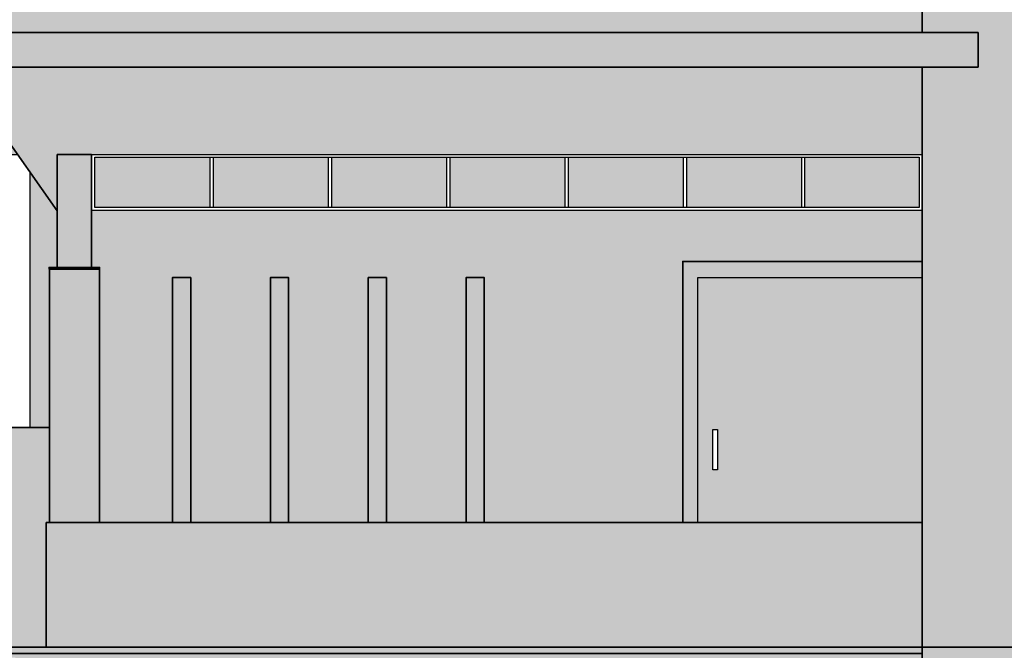
# Model space of a CAD drawing. Units: feet. Extents: x 2613 to 3913, y 950 to 1393.
# Tile 3 of 6: x 2725 to 2948, y 1083 to 1226. Entities that reach past the tile are written whole.
import ezdxf

# ---------------------------------------------------------------- set-up
doc = ezdxf.new("R2010")
doc.units = ezdxf.units.FT
for name, color, linetype, lineweight in [('A-DOOR', 3, 'Continuous', 25), ('A-ELEV', 7, 'Continuous', 35), ('A-ELEV-PATT', 9, 'Continuous', 13), ('A-GLAZ', 4, 'Continuous', 25)]:
    doc.layers.add(name, color=color, linetype=linetype, lineweight=lineweight)

msp = doc.modelspace()

# ---------------------------------------------------------------- hatches: boundary and pattern name
at = {"layer": 'A-ELEV-PATT'}
h = msp.add_hatch(color=256, dxfattribs=at)
h.dxf.hatch_style = 1
h.paths.add_polyline_path([(3108.91, 1328.81), (3061.44, 1376.28), (2929.45, 1244.29), (2929.45, 1223.38), (2942.09, 1223.38), (2942.09, 1215.5), (2929.45, 1215.5), (2929.45, 1084.12), (3108.91, 1084.12), (3108.91, 1199.69), (3106.87, 1199.69), (3106.87, 1128.72), (3017.91, 1128.72), (3017.91, 1199.69), (3008.08, 1199.69), (3008.08, 1180.01), (3007.65, 1180.01), (3007.65, 1199.69), (3004.75, 1199.69), (3004.75, 1206.47), (3108.91, 1206.47)])
h.paths.add_polyline_path([(3061.44, 1376.28), (3193.8, 1243.92), (3193.8, 1233.84), (3204.34, 1246.9), (3061.54, 1389.71), (2918.82, 1247), (2929.45, 1233.69), (2929.45, 1244.29)])
h.paths.add_polyline_path([(3061.54, 1389.71), (3204.34, 1246.9), (3206.69, 1248.02), (3061.63, 1393.09), (2916.59, 1248.06), (2918.82, 1247)])
h.paths.add_polyline_path([(2925.65, 1257.12), (2667.59, 1257.12), (2651.33, 1257.12), (2651.33, 1252.28), (2920.82, 1252.28)])
h.paths.add_polyline_path([(2920.82, 1252.28), (2651.33, 1252.28, -0.144454), (2652.15, 1251.12), (2667.59, 1251.12), (2919.65, 1251.12)])
h.paths.add_polyline_path([(2918.82, 1247), (2916.59, 1248.06), (2919.65, 1251.12), (2667.59, 1251.12), (2652.15, 1251.12), (2667.59, 1229.14), (2667.59, 1233.69), (2929.45, 1233.69)])
h.paths.add_polyline_path([(2710.6, 1223.38), (2929.45, 1223.38), (2929.45, 1233.69), (2667.59, 1233.69), (2667.59, 1229.14), (2667.59, 1201.16), (2720.67, 1201.16), (2710.6, 1215.5)])
h.paths.add_polyline_path([(2942.09, 1223.38), (2710.6, 1223.38), (2710.6, 1215.5), (2921.48, 1215.5), (2942.09, 1215.5)])
h.paths.add_polyline_path([(2929.45, 1215.5), (2921.48, 1215.5), (2710.6, 1215.5), (2733.47, 1182.94), (2733.47, 1195.74), (2741.22, 1195.74), (2929.45, 1195.74)])
h.paths.add_polyline_path([(2721, 1200.68), (2661.89, 1200.68), (2661.89, 1195.74), (2724.47, 1195.74)])
h.paths.add_polyline_path([(2733.47, 1182.94), (2727.27, 1191.76), (2727.27, 1133.88), (2731.7, 1133.88), (2731.7, 1169.74), (2731.61, 1169.74), (2731.61, 1170.13), (2733.47, 1170.13)])
h.paths.add_polyline_path([(2929.45, 1183.04), (2741.22, 1183.04), (2741.22, 1170.13), (2743.07, 1170.13), (2743.07, 1169.74), (2743.07, 1112.32), (2759.57, 1112.32), (2759.57, 1167.82), (2763.7, 1167.82), (2763.7, 1112.32), (2781.75, 1112.32), (2781.75, 1167.82), (2785.87, 1167.82), (2785.87, 1112.32), (2803.92, 1112.32), (2803.92, 1167.82), (2808.05, 1167.82), (2808.05, 1112.32), (2826.09, 1112.32), (2826.09, 1167.82), (2830.22, 1167.82), (2830.22, 1112.32), (2875.17, 1112.32), (2875.17, 1171.49), (2929.45, 1171.49)])
h.paths.add_polyline_path([(2731.7, 1133.88), (2661.89, 1133.88), (2661.89, 1084.12), (2730.99, 1084.12), (2730.99, 1112.32), (2731.7, 1112.32)])
h.paths.add_polyline_path([(2929.45, 1112.32), (2730.99, 1112.32), (2730.99, 1084.12), (2929.45, 1084.12)])
h.paths.add_polyline_path([(2929.45, 1084.12), (2730.99, 1084.12), (2661.89, 1084.12), (2612.72, 1084.12), (2612.72, 1082.68), (2929.45, 1082.68)])
h.paths.add_polyline_path([(2929.45, 1082.68), (2612.72, 1082.68), (2639.32, 1062.44), (2733.47, 1062.44), (2733.47, 1063.35), (2639.62, 1063.35), (2615.43, 1081.77), (2723.91, 1081.77), (2739.71, 1069.74), (2741.22, 1069.74), (2725.42, 1081.77), (2929.45, 1081.77)])
h.paths.add_polyline_path([(2671.42, 1081.77), (2668.07, 1081.77), (2692.27, 1063.35), (2695.62, 1063.35)], flags=17)
h.paths.add_polyline_path([(2741.22, 1069.74), (2741.22, 1068.59), (2748.11, 1063.35), (2741.22, 1063.35), (2741.22, 1062.44), (2750.82, 1062.44)], flags=17)
h.paths.add_polyline_path([(2929.45, 1081.77), (2725.42, 1081.77), (2750.82, 1062.44), (2741.22, 1062.44), (2741.22, 1047.95), (2743.07, 1047.95), (2743.07, 1047.56), (2743.07, 967.97), (2875.17, 967.97), (2875.17, 1066.37), (2929.45, 1066.37)])
h.paths.add_polyline_path([(2778.55, 1066.37), (2806.94, 1066.37), (2806.94, 982.04), (2778.55, 982.04)], flags=16)
h.paths.add_polyline_path([(2778.55, 1064.05), (2806.94, 1064.05), (2806.94, 1063.39), (2778.55, 1063.39)], flags=16)
h.paths.add_polyline_path([(2778.55, 1061.07), (2806.94, 1061.07), (2806.94, 1060.41), (2778.55, 1060.41)], flags=0)
h.paths.add_polyline_path([(2778.55, 1058.09), (2806.94, 1058.09), (2806.94, 1057.43), (2778.55, 1057.43)], flags=0)
h.paths.add_polyline_path([(2778.55, 1055.11), (2806.94, 1055.11), (2806.94, 1054.45), (2778.55, 1054.45)], flags=0)
h.paths.add_polyline_path([(2778.55, 1052.13), (2806.94, 1052.13), (2806.94, 1051.47), (2778.55, 1051.47)], flags=0)
h.paths.add_polyline_path([(2778.55, 1049.15), (2806.94, 1049.15), (2806.94, 1048.49), (2778.55, 1048.49)], flags=0)
h.paths.add_polyline_path([(2778.55, 1046.18), (2806.94, 1046.18), (2806.94, 1045.51), (2778.55, 1045.51)], flags=0)
h.paths.add_polyline_path([(2778.55, 1043.2), (2806.94, 1043.2), (2806.94, 1042.53), (2778.55, 1042.53)], flags=0)
h.paths.add_polyline_path([(2778.55, 1040.22), (2806.94, 1040.22), (2806.94, 1039.56), (2778.55, 1039.56)], flags=0)
h.paths.add_polyline_path([(2778.55, 1037.24), (2806.94, 1037.24), (2806.94, 1036.58), (2778.55, 1036.58)], flags=0)
h.paths.add_polyline_path([(2778.55, 1034.26), (2806.94, 1034.26), (2806.94, 1033.6), (2778.55, 1033.6)], flags=0)
h.paths.add_polyline_path([(2778.55, 1031.28), (2806.94, 1031.28), (2806.94, 1030.62), (2778.55, 1030.62)], flags=0)
h.paths.add_polyline_path([(2778.55, 1028.3), (2806.94, 1028.3), (2806.94, 1027.64), (2778.55, 1027.64)], flags=0)
h.paths.add_polyline_path([(2778.55, 1025.32), (2806.94, 1025.32), (2806.94, 1024.66), (2778.55, 1024.66)], flags=0)
h.paths.add_polyline_path([(2778.55, 1022.34), (2806.94, 1022.34), (2806.94, 1021.68), (2778.55, 1021.68)], flags=0)
h.paths.add_polyline_path([(2778.55, 1019.36), (2806.94, 1019.36), (2806.94, 1018.7), (2778.55, 1018.7)], flags=0)
h.paths.add_polyline_path([(2778.55, 1016.71), (2806.94, 1016.71), (2806.94, 1016.05), (2778.55, 1016.05)], flags=0)
h.paths.add_polyline_path([(2824.02, 1066.37), (2852.41, 1066.37), (2852.41, 982.04), (2824.02, 982.04)], flags=16)
h.paths.add_polyline_path([(2778.55, 1014.07), (2806.94, 1014.07), (2806.94, 1013.4), (2778.55, 1013.4)], flags=0)
h.paths.add_polyline_path([(2824.02, 1064.05), (2852.41, 1064.05), (2852.41, 1063.39), (2824.02, 1063.39)], flags=16)
h.paths.add_polyline_path([(2824.02, 1061.07), (2852.41, 1061.07), (2852.41, 1060.41), (2824.02, 1060.41)], flags=0)
h.paths.add_polyline_path([(2824.02, 1058.09), (2852.41, 1058.09), (2852.41, 1057.43), (2824.02, 1057.43)], flags=0)
h.paths.add_polyline_path([(2824.02, 1055.11), (2852.41, 1055.11), (2852.41, 1054.45), (2824.02, 1054.45)], flags=16)
h.paths.add_polyline_path([(2824.02, 1052.13), (2852.41, 1052.13), (2852.41, 1051.47), (2824.02, 1051.47)], flags=0)
h.paths.add_polyline_path([(2778.55, 1011.09), (2806.94, 1011.09), (2806.94, 1010.43), (2778.55, 1010.43)], flags=0)
h.paths.add_polyline_path([(2824.02, 1049.15), (2852.41, 1049.15), (2852.41, 1048.49), (2824.02, 1048.49)], flags=0)
h.paths.add_polyline_path([(2824.02, 1046.18), (2852.41, 1046.18), (2852.41, 1045.51), (2824.02, 1045.51)], flags=0)
h.paths.add_polyline_path([(2824.02, 1043.2), (2852.41, 1043.2), (2852.41, 1042.53), (2824.02, 1042.53)], flags=0)
h.paths.add_polyline_path([(2778.55, 1008.11), (2806.94, 1008.11), (2806.94, 1007.45), (2778.55, 1007.45)], flags=0)
h.paths.add_polyline_path([(2824.02, 1040.22), (2852.41, 1040.22), (2852.41, 1039.56), (2824.02, 1039.56)], flags=0)
h.paths.add_polyline_path([(2824.02, 1037.24), (2852.41, 1037.24), (2852.41, 1036.58), (2824.02, 1036.58)], flags=0)
h.paths.add_polyline_path([(2778.55, 1005.13), (2806.94, 1005.13), (2806.94, 1004.47), (2778.55, 1004.47)], flags=0)
h.paths.add_polyline_path([(2824.02, 1034.26), (2852.41, 1034.26), (2852.41, 1033.6), (2824.02, 1033.6)], flags=0)
h.paths.add_polyline_path([(2824.02, 1031.28), (2852.41, 1031.28), (2852.41, 1030.62), (2824.02, 1030.62)], flags=0)
h.paths.add_polyline_path([(2778.55, 1002.15), (2806.94, 1002.15), (2806.94, 1001.49), (2778.55, 1001.49)], flags=0)
h.paths.add_polyline_path([(2824.02, 1028.3), (2852.41, 1028.3), (2852.41, 1027.64), (2824.02, 1027.64)], flags=0)
h.paths.add_polyline_path([(2778.55, 999.17), (2806.94, 999.17), (2806.94, 998.51), (2778.55, 998.51)], flags=0)
h.paths.add_polyline_path([(2824.02, 1025.32), (2852.41, 1025.32), (2852.41, 1024.66), (2824.02, 1024.66)], flags=0)
h.paths.add_polyline_path([(2824.02, 1022.34), (2852.41, 1022.34), (2852.41, 1021.68), (2824.02, 1021.68)], flags=0)
h.paths.add_polyline_path([(2778.55, 996.19), (2806.94, 996.19), (2806.94, 995.53), (2778.55, 995.53)], flags=0)
h.paths.add_polyline_path([(2824.02, 1019.36), (2852.41, 1019.36), (2852.41, 1018.7), (2824.02, 1018.7)], flags=0)
h.paths.add_polyline_path([(2778.55, 993.21), (2806.94, 993.21), (2806.94, 992.55), (2778.55, 992.55)], flags=0)
h.paths.add_polyline_path([(2824.02, 1016.38), (2852.41, 1016.38), (2852.41, 1015.72), (2824.02, 1015.72)], flags=0)
h.paths.add_polyline_path([(2824.02, 1013.4), (2852.41, 1013.4), (2852.41, 1012.74), (2824.02, 1012.74)], flags=0)
h.paths.add_polyline_path([(2778.55, 990.23), (2806.94, 990.23), (2806.94, 989.57), (2778.55, 989.57)], flags=0)
h.paths.add_polyline_path([(2824.02, 1010.43), (2852.41, 1010.43), (2852.41, 1009.76), (2824.02, 1009.76)], flags=0)
h.paths.add_polyline_path([(2778.55, 987.25), (2806.94, 987.25), (2806.94, 986.59), (2778.55, 986.59)], flags=0)
h.paths.add_polyline_path([(2824.02, 1007.45), (2852.41, 1007.45), (2852.41, 1006.78), (2824.02, 1006.78)], flags=0)
h.paths.add_polyline_path([(2778.55, 984.27), (2806.94, 984.27), (2806.94, 983.61), (2778.55, 983.61)], flags=0)
h.paths.add_polyline_path([(2824.02, 1004.47), (2852.41, 1004.47), (2852.41, 1003.81), (2824.02, 1003.81)], flags=0)
h.paths.add_polyline_path([(2824.02, 1001.49), (2852.41, 1001.49), (2852.41, 1000.83), (2824.02, 1000.83)], flags=0)
h.paths.add_polyline_path([(2824.02, 998.51), (2852.41, 998.51), (2852.41, 997.85), (2824.02, 997.85)], flags=0)
h.paths.add_polyline_path([(2824.02, 995.53), (2852.41, 995.53), (2852.41, 994.87), (2824.02, 994.87)], flags=0)
h.paths.add_polyline_path([(2824.02, 992.55), (2852.41, 992.55), (2852.41, 991.89), (2824.02, 991.89)], flags=0)
h.paths.add_polyline_path([(2824.02, 989.57), (2852.41, 989.57), (2852.41, 988.91), (2824.02, 988.91)], flags=0)
h.paths.add_polyline_path([(2824.02, 986.59), (2852.41, 986.59), (2852.41, 985.93), (2824.02, 985.93)], flags=0)
h.paths.add_polyline_path([(2824.02, 983.61), (2852.41, 983.61), (2852.41, 982.95), (2824.02, 982.95)], flags=0)
h.paths.add_polyline_path([(2731.7, 1047.56), (2731.61, 1047.56), (2731.61, 1047.95), (2733.47, 1047.95), (2733.47, 1062.44), (2727.27, 1062.44), (2727.27, 1000.58), (2667.59, 1000.58), (2667.59, 1062.44), (2664.87, 1062.44), (2664.87, 965.01), (2730.76, 964.93), (2730.76, 967.97), (2731.7, 967.97)])
h.paths.add_polyline_path([(2728.06, 961.9), (2730.76, 961.9), (2730.76, 964.93), (2663.94, 964.93), (2663.94, 949.74), (2725.36, 949.74), (2725.36, 955.82), (2728.06, 955.82)])
h.paths.add_polyline_path([(2929.45, 967.97), (2730.76, 967.97), (2730.76, 961.9), (2929.45, 961.9)])
h.paths.add_polyline_path([(2929.45, 961.9), (2730.76, 961.9), (2728.06, 961.9), (2728.06, 955.82), (2929.45, 955.82)])
h.paths.add_polyline_path([(2929.45, 955.82), (2728.06, 955.82), (2725.36, 955.82), (2725.36, 949.74), (2929.45, 949.74)])
h.paths.add_polyline_path([(2741.22, 1069.74), (2733.47, 1069.74), (2733.47, 1047.95), (2741.22, 1047.95)], flags=17)
h.paths.add_polyline_path([(2741.22, 1195.74), (2733.47, 1195.74), (2733.47, 1182.94), (2733.47, 1170.13), (2741.22, 1170.13), (2741.22, 1183.04)])
h.paths.add_polyline_path([(3193.8, 1084.12), (2929.45, 1084.12), (2929.45, 1082.68), (2929.45, 1081.77), (2929.45, 1066.37), (2929.45, 949.74), (3193.8, 949.74)])
h.paths.add_polyline_path([(2937.79, 1075.78), (3185.46, 1075.78), (3185.46, 958.09), (2937.79, 958.09)], flags=16)
h.paths.add_polyline_path([(3011.76, 1075.78), (3104.46, 1075.78), (3104.46, 993.6), (3011.76, 993.6)], flags=0)
h.paths.add_polyline_path([(3015.24, 1075.78), (3016.57, 1075.78), (3016.57, 1060.85), (3043.1, 1060.85), (3043.1, 1075.78), (3045.77, 1075.78), (3045.77, 997.08), (3070.45, 997.08), (3070.45, 1075.78), (3073.12, 1075.78), (3073.12, 1060.85), (3099.64, 1060.85), (3099.64, 1075.78), (3100.98, 1075.78), (3100.98, 997.08), (3099.64, 997.08), (3015.24, 997.08)], flags=0)
h = msp.add_hatch(color=256, dxfattribs=at)
h.dxf.hatch_style = 1
h.paths.add_polyline_path([(2768.1, 1195.09), (2741.95, 1195.09), (2741.95, 1183.7), (2768.1, 1183.7)])
h.paths.add_polyline_path([(2794.91, 1195.09), (2768.76, 1195.09), (2768.76, 1183.7), (2794.91, 1183.7)])
h.paths.add_polyline_path([(2821.72, 1195.09), (2795.57, 1195.09), (2795.57, 1183.7), (2821.72, 1183.7)])
h.paths.add_polyline_path([(2848.53, 1195.09), (2822.38, 1195.09), (2822.38, 1183.7), (2848.53, 1183.7)])
h.paths.add_polyline_path([(2875.34, 1195.09), (2849.19, 1195.09), (2849.19, 1183.7), (2875.34, 1183.7)])
h.paths.add_polyline_path([(2683.29, 1193.04), (2670.29, 1193.04), (2670.29, 1190.17), (2683.29, 1190.17)])
h.paths.add_polyline_path([(2696.31, 1193.04), (2683.32, 1193.04), (2683.32, 1190.17), (2696.31, 1190.17)])
h.paths.add_polyline_path([(2696.31, 1190.14), (2683.32, 1190.14), (2683.32, 1187.27), (2696.31, 1187.27)])
h.paths.add_polyline_path([(2683.29, 1190.14), (2670.29, 1190.14), (2670.29, 1187.27), (2683.29, 1187.27)])
h.paths.add_polyline_path([(2683.29, 1187.24), (2670.29, 1187.24), (2670.29, 1184.37), (2683.29, 1184.37)])
h.paths.add_polyline_path([(2696.31, 1187.24), (2683.32, 1187.24), (2683.32, 1184.37), (2696.31, 1184.37)])
h.paths.add_polyline_path([(2683.29, 1184.34), (2670.29, 1184.34), (2670.29, 1181.47), (2683.29, 1181.47)])
h.paths.add_polyline_path([(2696.31, 1184.34), (2683.32, 1184.34), (2683.32, 1181.47), (2696.31, 1181.47)])
h.paths.add_polyline_path([(2683.29, 1181.44), (2670.29, 1181.44), (2670.29, 1178.57), (2683.29, 1178.57)])
h.paths.add_polyline_path([(2696.31, 1181.44), (2683.32, 1181.44), (2683.32, 1178.57), (2696.31, 1178.57)])
h.paths.add_polyline_path([(2696.31, 1178.53), (2683.32, 1178.53), (2683.32, 1175.67), (2696.31, 1175.67)])
h.paths.add_polyline_path([(2683.29, 1178.53), (2670.29, 1178.53), (2670.29, 1175.67), (2683.29, 1175.67)])
h.paths.add_polyline_path([(2683.29, 1175.63), (2670.29, 1175.63), (2670.29, 1172.76), (2683.29, 1172.76)])
h.paths.add_polyline_path([(2696.31, 1175.63), (2683.32, 1175.63), (2683.32, 1172.76), (2696.31, 1172.76)])
h.paths.add_polyline_path([(2683.29, 1172.73), (2670.29, 1172.73), (2670.29, 1169.86), (2683.29, 1169.86)])
h.paths.add_polyline_path([(2696.31, 1172.73), (2683.32, 1172.73), (2683.32, 1169.86), (2696.31, 1169.86)])
h.paths.add_polyline_path([(2696.31, 1169.83), (2683.32, 1169.83), (2683.32, 1166.96), (2696.31, 1166.96)])
h.paths.add_polyline_path([(2683.29, 1169.83), (2670.29, 1169.83), (2670.29, 1166.96), (2683.29, 1166.96)])
h.paths.add_polyline_path([(2696.31, 1166.93), (2683.32, 1166.93), (2683.32, 1164.06), (2696.31, 1164.06)])
h.paths.add_polyline_path([(2683.29, 1166.93), (2670.29, 1166.93), (2670.29, 1164.06), (2683.29, 1164.06)])
h.paths.add_polyline_path([(2683.29, 1164.03), (2670.29, 1164.03), (2670.29, 1161.16), (2683.29, 1161.16)])
h.paths.add_polyline_path([(2696.31, 1164.03), (2683.32, 1164.03), (2683.32, 1161.16), (2696.31, 1161.16)])
h.paths.add_polyline_path([(2696.31, 1161.12), (2683.32, 1161.12), (2683.32, 1158.25), (2696.31, 1158.25)])
h.paths.add_polyline_path([(2683.29, 1161.12), (2670.29, 1161.12), (2670.29, 1158.25), (2683.29, 1158.25)])
h.paths.add_polyline_path([(2683.29, 1158.22), (2670.29, 1158.22), (2670.29, 1155.35), (2683.29, 1155.35)])
h.paths.add_polyline_path([(2696.31, 1158.22), (2683.32, 1158.22), (2683.32, 1155.35), (2696.31, 1155.35)])
h.paths.add_polyline_path([(2696.31, 1155.32), (2683.32, 1155.32), (2683.32, 1152.45), (2696.31, 1152.45)])
h.paths.add_polyline_path([(2683.29, 1155.32), (2670.29, 1155.32), (2670.29, 1152.45), (2683.29, 1152.45)])
h.paths.add_polyline_path([(2683.29, 1152.42), (2670.29, 1152.42), (2670.29, 1149.55), (2683.29, 1149.55)])
h.paths.add_polyline_path([(2696.31, 1152.42), (2683.32, 1152.42), (2683.32, 1149.55), (2696.31, 1149.55)])
h.paths.add_polyline_path([(2683.29, 1149.52), (2670.29, 1149.52), (2670.29, 1146.65), (2683.29, 1146.65)])
h.paths.add_polyline_path([(2696.31, 1149.52), (2683.32, 1149.52), (2683.32, 1146.65), (2696.31, 1146.65)])
h.paths.add_polyline_path([(2696.31, 1146.61), (2683.32, 1146.61), (2683.32, 1143.75), (2696.31, 1143.75)])
h.paths.add_polyline_path([(2683.29, 1146.61), (2670.29, 1146.61), (2670.29, 1143.75), (2683.29, 1143.75)])
h.paths.add_polyline_path([(2683.29, 1143.71), (2670.29, 1143.71), (2670.29, 1140.84), (2683.29, 1140.84)])
h.paths.add_polyline_path([(2696.31, 1143.71), (2683.32, 1143.71), (2683.32, 1140.84), (2696.31, 1140.84)])
h.paths.add_polyline_path([(2683.29, 1140.81), (2670.29, 1140.81), (2670.29, 1137.94), (2683.29, 1137.94)])
h.paths.add_polyline_path([(2696.31, 1140.81), (2683.32, 1140.81), (2683.32, 1137.94), (2696.31, 1137.94)])
h.paths.add_polyline_path([(2683.29, 1137.91), (2670.29, 1137.91), (2670.29, 1136.58), (2683.29, 1136.58)])
h.paths.add_polyline_path([(2696.31, 1137.91), (2683.32, 1137.91), (2683.32, 1136.58), (2696.31, 1136.58)])
h.paths.add_polyline_path([(3074.7, 1198.4), (3050.02, 1198.4), (3050.02, 1130.01), (3074.7, 1130.01)])
h.paths.add_polyline_path([(3047.34, 1198.4), (3019.29, 1198.4), (3019.29, 1184.76), (3047.34, 1184.76)])
h.paths.add_polyline_path([(3047.34, 1183.78), (3019.29, 1183.78), (3019.29, 1130.01), (3047.34, 1130.01)])
h.paths.add_polyline_path([(3105.48, 1198.4), (3077.37, 1198.4), (3077.37, 1184.76), (3105.48, 1184.76)])
h.paths.add_polyline_path([(3105.48, 1183.78), (3077.37, 1183.78), (3077.37, 1130.01), (3105.48, 1130.01)])
h.paths.add_polyline_path([(3070.45, 1075.78), (3045.77, 1075.78), (3045.77, 997.08), (3070.45, 997.08)])
h.paths.add_polyline_path([(3099.64, 1075.78), (3073.12, 1075.78), (3073.12, 1060.85), (3099.64, 1060.85)])
h.paths.add_polyline_path([(3099.64, 1059.87), (3073.12, 1059.87), (3073.12, 997.08), (3099.64, 997.08)])
h.paths.add_polyline_path([(3043.1, 1075.78), (3016.57, 1075.78), (3016.57, 1060.85), (3043.1, 1060.85)])
h.paths.add_polyline_path([(3043.1, 1059.87), (3016.57, 1059.87), (3016.57, 997.08), (3043.1, 997.08)])
h.paths.add_polyline_path([(2683.29, 1059.73), (2670.29, 1059.73), (2670.29, 1056.87), (2683.29, 1056.87)])
h.paths.add_polyline_path([(2696.31, 1059.73), (2683.32, 1059.73), (2683.32, 1056.87), (2696.31, 1056.87)])
h.paths.add_polyline_path([(2696.31, 1056.83), (2683.32, 1056.83), (2683.32, 1053.96), (2696.31, 1053.96)])
h.paths.add_polyline_path([(2683.29, 1056.83), (2670.29, 1056.83), (2670.29, 1053.96), (2683.29, 1053.96)])
h.paths.add_polyline_path([(2683.29, 1053.93), (2670.29, 1053.93), (2670.29, 1051.06), (2683.29, 1051.06)])
h.paths.add_polyline_path([(2696.31, 1053.93), (2683.32, 1053.93), (2683.32, 1051.06), (2696.31, 1051.06)])
h.paths.add_polyline_path([(2683.29, 1051.03), (2670.29, 1051.03), (2670.29, 1048.16), (2683.29, 1048.16)])
h.paths.add_polyline_path([(2696.31, 1051.03), (2683.32, 1051.03), (2683.32, 1048.16), (2696.31, 1048.16)])
h.paths.add_polyline_path([(2683.29, 1048.13), (2670.29, 1048.13), (2670.29, 1045.26), (2683.29, 1045.26)])
h.paths.add_polyline_path([(2696.31, 1048.13), (2683.32, 1048.13), (2683.32, 1045.26), (2696.31, 1045.26)])
h.paths.add_polyline_path([(2696.31, 1045.23), (2683.32, 1045.23), (2683.32, 1042.36), (2696.31, 1042.36)])
h.paths.add_polyline_path([(2683.29, 1045.23), (2670.29, 1045.23), (2670.29, 1042.36), (2683.29, 1042.36)])
h.paths.add_polyline_path([(2683.29, 1042.32), (2670.29, 1042.32), (2670.29, 1039.46), (2683.29, 1039.46)])
h.paths.add_polyline_path([(2696.31, 1042.32), (2683.32, 1042.32), (2683.32, 1039.46), (2696.31, 1039.46)])
h.paths.add_polyline_path([(2696.31, 1039.42), (2683.32, 1039.42), (2683.32, 1036.55), (2696.31, 1036.55)])
h.paths.add_polyline_path([(2683.29, 1039.42), (2670.29, 1039.42), (2670.29, 1036.55), (2683.29, 1036.55)])
h.paths.add_polyline_path([(2683.29, 1036.52), (2670.29, 1036.52), (2670.29, 1033.65), (2683.29, 1033.65)])
h.paths.add_polyline_path([(2696.31, 1036.52), (2683.32, 1036.52), (2683.32, 1033.65), (2696.31, 1033.65)])
h.paths.add_polyline_path([(2696.31, 1033.62), (2683.32, 1033.62), (2683.32, 1030.75), (2696.31, 1030.75)])
h.paths.add_polyline_path([(2683.29, 1033.62), (2670.29, 1033.62), (2670.29, 1030.75), (2683.29, 1030.75)])
h.paths.add_polyline_path([(2696.31, 1030.72), (2683.32, 1030.72), (2683.32, 1027.85), (2696.31, 1027.85)])
h.paths.add_polyline_path([(2683.29, 1030.72), (2670.29, 1030.72), (2670.29, 1027.85), (2683.29, 1027.85)])
h.paths.add_polyline_path([(2683.29, 1027.82), (2670.29, 1027.82), (2670.29, 1024.95), (2683.29, 1024.95)])
h.paths.add_polyline_path([(2696.31, 1027.82), (2683.32, 1027.82), (2683.32, 1024.95), (2696.31, 1024.95)])
h.paths.add_polyline_path([(2696.31, 1024.91), (2683.32, 1024.91), (2683.32, 1022.05), (2696.31, 1022.05)])
h.paths.add_polyline_path([(2683.29, 1024.91), (2670.29, 1024.91), (2670.29, 1022.05), (2683.29, 1022.05)])
h.paths.add_polyline_path([(2683.29, 1022.01), (2670.29, 1022.01), (2670.29, 1019.14), (2683.29, 1019.14)])
h.paths.add_polyline_path([(2696.31, 1022.01), (2683.32, 1022.01), (2683.32, 1019.14), (2696.31, 1019.14)])
h.paths.add_polyline_path([(2696.31, 1019.11), (2683.32, 1019.11), (2683.32, 1016.24), (2696.31, 1016.24)])
h.paths.add_polyline_path([(2683.29, 1019.11), (2670.29, 1019.11), (2670.29, 1016.24), (2683.29, 1016.24)])
h.paths.add_polyline_path([(2683.29, 1016.21), (2670.29, 1016.21), (2670.29, 1013.34), (2683.29, 1013.34)])
h.paths.add_polyline_path([(2696.31, 1016.21), (2683.32, 1016.21), (2683.32, 1013.34), (2696.31, 1013.34)])
h.paths.add_polyline_path([(2696.31, 1013.31), (2683.32, 1013.31), (2683.32, 1010.44), (2696.31, 1010.44)])
h.paths.add_polyline_path([(2683.29, 1013.31), (2670.29, 1013.31), (2670.29, 1010.44), (2683.29, 1010.44)])
h.paths.add_polyline_path([(2683.29, 1010.41), (2670.29, 1010.41), (2670.29, 1007.54), (2683.29, 1007.54)])
h.paths.add_polyline_path([(2696.31, 1010.41), (2683.32, 1010.41), (2683.32, 1007.54), (2696.31, 1007.54)])
h.paths.add_polyline_path([(2696.31, 1007.5), (2683.32, 1007.5), (2683.32, 1004.64), (2696.31, 1004.64)])
h.paths.add_polyline_path([(2683.29, 1007.5), (2670.29, 1007.5), (2670.29, 1004.64), (2683.29, 1004.64)])
h.paths.add_polyline_path([(2683.29, 1004.6), (2670.29, 1004.6), (2670.29, 1003.28), (2683.29, 1003.28)])
h.paths.add_polyline_path([(2696.31, 1004.6), (2683.32, 1004.6), (2683.32, 1003.28), (2696.31, 1003.28)])
h.paths.add_polyline_path([(2806.94, 1066.37), (2778.55, 1066.37), (2778.55, 1064.05), (2806.94, 1064.05)])
h.paths.add_polyline_path([(2806.94, 1063.39), (2778.55, 1063.39), (2778.55, 1061.07), (2806.94, 1061.07)])
h.paths.add_polyline_path([(2806.94, 1060.41), (2778.55, 1060.41), (2778.55, 1058.09), (2806.94, 1058.09)])
h.paths.add_polyline_path([(2806.94, 1057.43), (2778.55, 1057.43), (2778.55, 1055.11), (2806.94, 1055.11)])
h.paths.add_polyline_path([(2806.94, 1054.45), (2778.55, 1054.45), (2778.55, 1052.13), (2806.94, 1052.13)])
h.paths.add_polyline_path([(2806.94, 1051.47), (2778.55, 1051.47), (2778.55, 1049.15), (2806.94, 1049.15)])
h.paths.add_polyline_path([(2806.94, 1048.49), (2778.55, 1048.49), (2778.55, 1046.18), (2806.94, 1046.18)])
h.paths.add_polyline_path([(2806.94, 1045.51), (2778.55, 1045.51), (2778.55, 1043.2), (2806.94, 1043.2)])
h.paths.add_polyline_path([(2806.94, 1042.53), (2778.55, 1042.53), (2778.55, 1040.22), (2806.94, 1040.22)])
h.paths.add_polyline_path([(2806.94, 1039.56), (2778.55, 1039.56), (2778.55, 1037.24), (2806.94, 1037.24)])
h.paths.add_polyline_path([(2806.94, 1036.58), (2778.55, 1036.58), (2778.55, 1034.26), (2806.94, 1034.26)])
h.paths.add_polyline_path([(2806.94, 1033.6), (2778.55, 1033.6), (2778.55, 1031.28), (2806.94, 1031.28)])
h.paths.add_polyline_path([(2806.94, 1030.62), (2778.55, 1030.62), (2778.55, 1028.3), (2806.94, 1028.3)])
h.paths.add_polyline_path([(2806.94, 1027.64), (2778.55, 1027.64), (2778.55, 1025.32), (2806.94, 1025.32)])
h.paths.add_polyline_path([(2806.94, 1024.66), (2778.55, 1024.66), (2778.55, 1022.34), (2806.94, 1022.34)])
h.paths.add_polyline_path([(2806.94, 1021.68), (2778.55, 1021.68), (2778.55, 1019.36), (2806.94, 1019.36)])
h.paths.add_polyline_path([(2806.94, 1018.7), (2778.55, 1018.7), (2778.55, 1016.71), (2806.94, 1016.71)])
h.paths.add_polyline_path([(2806.94, 1016.05), (2778.55, 1016.05), (2778.55, 1014.07), (2806.94, 1014.07)])
h.paths.add_polyline_path([(2806.94, 1013.4), (2778.55, 1013.4), (2778.55, 1011.09), (2806.94, 1011.09)])
h.paths.add_polyline_path([(2806.94, 1010.43), (2778.55, 1010.43), (2778.55, 1008.11), (2806.94, 1008.11)])
h.paths.add_polyline_path([(2806.94, 1007.45), (2778.55, 1007.45), (2778.55, 1005.13), (2806.94, 1005.13)])
h.paths.add_polyline_path([(2806.94, 1004.47), (2778.55, 1004.47), (2778.55, 1002.15), (2806.94, 1002.15)])
h.paths.add_polyline_path([(2806.94, 1001.49), (2778.55, 1001.49), (2778.55, 999.17), (2806.94, 999.17)])
h.paths.add_polyline_path([(2806.94, 998.51), (2778.55, 998.51), (2778.55, 996.19), (2806.94, 996.19)])
h.paths.add_polyline_path([(2806.94, 983.61), (2778.55, 983.61), (2778.55, 982.04), (2806.94, 982.04)])
h.paths.add_polyline_path([(2806.94, 986.59), (2778.55, 986.59), (2778.55, 984.27), (2806.94, 984.27)])
h.paths.add_polyline_path([(2806.94, 989.57), (2778.55, 989.57), (2778.55, 987.25), (2806.94, 987.25)])
h.paths.add_polyline_path([(2806.94, 992.55), (2778.55, 992.55), (2778.55, 990.23), (2806.94, 990.23)])
h.paths.add_polyline_path([(2806.94, 995.53), (2778.55, 995.53), (2778.55, 993.21), (2806.94, 993.21)])
h.paths.add_polyline_path([(2852.41, 985.93), (2824.02, 985.93), (2824.02, 983.61), (2852.41, 983.61)])
h.paths.add_polyline_path([(2852.41, 982.95), (2824.02, 982.95), (2824.02, 982.04), (2852.41, 982.04)])
h.paths.add_polyline_path([(2852.41, 988.91), (2824.02, 988.91), (2824.02, 986.59), (2852.41, 986.59)])
h.paths.add_polyline_path([(2852.41, 991.89), (2824.02, 991.89), (2824.02, 989.57), (2852.41, 989.57)])
h.paths.add_polyline_path([(2852.41, 994.87), (2824.02, 994.87), (2824.02, 992.55), (2852.41, 992.55)])
h.paths.add_polyline_path([(2852.41, 997.85), (2824.02, 997.85), (2824.02, 995.53), (2852.41, 995.53)])
h.paths.add_polyline_path([(2852.41, 1000.83), (2824.02, 1000.83), (2824.02, 998.51), (2852.41, 998.51)])
h.paths.add_polyline_path([(2852.41, 1003.81), (2824.02, 1003.81), (2824.02, 1001.49), (2852.41, 1001.49)])
h.paths.add_polyline_path([(2852.41, 1006.78), (2824.02, 1006.78), (2824.02, 1004.47), (2852.41, 1004.47)])
h.paths.add_polyline_path([(2852.41, 1009.76), (2824.02, 1009.76), (2824.02, 1007.45), (2852.41, 1007.45)])
h.paths.add_polyline_path([(2852.41, 1012.74), (2824.02, 1012.74), (2824.02, 1010.43), (2852.41, 1010.43)])
h.paths.add_polyline_path([(2852.41, 1015.72), (2824.02, 1015.72), (2824.02, 1013.4), (2852.41, 1013.4)])
h.paths.add_polyline_path([(2852.41, 1018.7), (2824.02, 1018.7), (2824.02, 1016.38), (2852.41, 1016.38)])
h.paths.add_polyline_path([(2852.41, 1021.68), (2824.02, 1021.68), (2824.02, 1019.36), (2852.41, 1019.36)])
h.paths.add_polyline_path([(2852.41, 1024.66), (2824.02, 1024.66), (2824.02, 1022.34), (2852.41, 1022.34)])
h.paths.add_polyline_path([(2852.41, 1027.64), (2824.02, 1027.64), (2824.02, 1025.32), (2852.41, 1025.32)])
h.paths.add_polyline_path([(2852.41, 1030.62), (2824.02, 1030.62), (2824.02, 1028.3), (2852.41, 1028.3)])
h.paths.add_polyline_path([(2852.41, 1033.6), (2824.02, 1033.6), (2824.02, 1031.28), (2852.41, 1031.28)])
h.paths.add_polyline_path([(2852.41, 1036.58), (2824.02, 1036.58), (2824.02, 1034.26), (2852.41, 1034.26)])
h.paths.add_polyline_path([(2852.41, 1039.56), (2824.02, 1039.56), (2824.02, 1037.24), (2852.41, 1037.24)])
h.paths.add_polyline_path([(2852.41, 1042.53), (2824.02, 1042.53), (2824.02, 1040.22), (2852.41, 1040.22)])
h.paths.add_polyline_path([(2852.41, 1045.51), (2824.02, 1045.51), (2824.02, 1043.2), (2852.41, 1043.2)])
h.paths.add_polyline_path([(2852.41, 1048.49), (2824.02, 1048.49), (2824.02, 1046.18), (2852.41, 1046.18)])
h.paths.add_polyline_path([(2852.41, 1066.37), (2824.02, 1066.37), (2824.02, 1049.15), (2852.41, 1049.15)])
h = msp.add_hatch(color=256, dxfattribs=at)
h.dxf.hatch_style = 1
h.paths.add_polyline_path([(2902.15, 1195.09), (2876, 1195.09), (2876, 1183.7), (2902.15, 1183.7)])
h.paths.add_polyline_path([(2928.72, 1195.09), (2902.8, 1195.09), (2902.8, 1183.7), (2928.72, 1183.7)])
h.paths.add_polyline_path([(2830.22, 1167.82), (2826.09, 1167.82), (2826.09, 1112.32), (2830.22, 1112.32)])
h.paths.add_polyline_path([(2808.05, 1167.82), (2803.92, 1167.82), (2803.92, 1112.32), (2808.05, 1112.32)])
h.paths.add_polyline_path([(2785.87, 1167.82), (2781.75, 1167.82), (2781.75, 1112.32), (2785.87, 1112.32)])
h.paths.add_polyline_path([(2763.7, 1167.82), (2759.57, 1167.82), (2759.57, 1112.32), (2763.7, 1112.32)])
h = msp.add_hatch(color=256, dxfattribs=at)
h.dxf.hatch_style = 1
h.paths.add_polyline_path([(2929.45, 1167.82), (2878.62, 1167.82), (2878.62, 1112.32), (2929.45, 1112.32)], flags=17)
h.paths.add_polyline_path([(2883.07, 1133.45), (2883.07, 1124.29), (2881.96, 1124.29), (2881.96, 1133.45)], flags=16)
h.paths.add_polyline_path([(2929.45, 1171.49), (2875.17, 1171.49), (2875.17, 1112.32), (2878.62, 1112.32), (2878.62, 1167.82), (2929.45, 1167.82)])
h.paths.add_polyline_path([(2929.45, 1062.69), (2878.62, 1062.69), (2878.62, 967.97), (2929.45, 967.97)], flags=17)
h.paths.add_polyline_path([(2883.07, 1020.32), (2883.07, 1011.16), (2881.96, 1011.16), (2881.96, 1020.32)], flags=16)
h.paths.add_polyline_path([(2929.45, 1066.37), (2875.17, 1066.37), (2875.17, 967.97), (2878.62, 967.97), (2878.62, 1062.69), (2929.45, 1062.69)])
h.paths.add_polyline_path([(3011.76, 1075.78), (2937.79, 1075.78), (2937.79, 958.09), (3185.46, 958.09), (3185.46, 1075.78), (3104.46, 1075.78), (3104.46, 993.6), (3011.76, 993.6)])
h = msp.add_hatch(color=256, dxfattribs=at)
h.dxf.hatch_style = 1
h.paths.add_polyline_path([(2743.07, 1169.74), (2731.7, 1169.74), (2731.7, 1112.32), (2743.07, 1112.32)])
h.paths.add_polyline_path([(2743.07, 1047.56), (2731.7, 1047.56), (2731.7, 967.97), (2743.07, 967.97)])

# ---------------------------------------------------------------- linework, layer by layer
at = {"layer": 'A-DOOR'}
msp.add_lwpolyline([(2878.62, 1112.32), (2878.62, 1167.82), (2929.45, 1167.82), (2929.45, 1112.32)], dxfattribs=at)
msp.add_lwpolyline([(2878.62, 1112.32), (2878.62, 1167.82), (2929.45, 1167.82), (2929.45, 1112.32)], dxfattribs=at)
msp.add_lwpolyline([(2881.96, 1133.45), (2883.07, 1133.45), (2883.07, 1124.29), (2881.96, 1124.29)], close=True, dxfattribs=at)
msp.add_lwpolyline([(2881.96, 1133.45), (2883.07, 1133.45), (2883.07, 1124.29), (2881.96, 1124.29)], close=True, dxfattribs=at)
at = {"layer": 'A-ELEV'}
for p, q in [((2942.09, 1223.38), (2710.6, 1223.38)), ((2942.09, 1223.38), (2710.6, 1223.38)), ((2942.09, 1215.5), (2942.09, 1223.38)), ((2942.09, 1215.5), (2942.09, 1223.38)), ((2733.47, 1182.94), (2710.6, 1215.5)), ((2710.6, 1215.5), (2921.48, 1215.5)), ((2733.47, 1182.94), (2710.6, 1215.5)), ((2710.6, 1215.5), (2921.48, 1215.5)), ((2921.48, 1215.5), (2942.09, 1215.5)), ((2921.48, 1215.5), (2942.09, 1215.5))]:
    msp.add_line(p, q, dxfattribs=at)
for points in [[(2929.45, 1244.29), (2929.45, 1223.38)], [(2929.45, 1244.29), (2929.45, 1223.38)], [(2929.45, 1215.5), (2929.45, 1084.12)], [(2929.45, 1215.5), (2929.45, 1084.12)], [(2875.17, 1112.32), (2875.17, 1171.49), (2929.45, 1171.49), (2929.45, 1112.32)], [(2875.17, 1112.32), (2875.17, 1171.49), (2929.45, 1171.49), (2929.45, 1112.32)], [(2731.7, 1112.32), (2731.7, 1169.74), (2743.07, 1169.74), (2743.07, 1112.32)], [(2731.7, 1112.32), (2731.7, 1169.74), (2743.07, 1169.74), (2743.07, 1112.32)], [(2763.7, 1112.32), (2763.7, 1167.82), (2759.57, 1167.82), (2759.57, 1112.32)], [(2763.7, 1112.32), (2763.7, 1167.82), (2759.57, 1167.82), (2759.57, 1112.32)], [(2785.87, 1112.32), (2785.87, 1167.82), (2781.75, 1167.82), (2781.75, 1112.32)], [(2785.87, 1112.32), (2785.87, 1167.82), (2781.75, 1167.82), (2781.75, 1112.32)], [(2808.05, 1112.32), (2808.05, 1167.82), (2803.92, 1167.82), (2803.92, 1112.32)], [(2808.05, 1112.32), (2808.05, 1167.82), (2803.92, 1167.82), (2803.92, 1112.32)], [(2830.22, 1112.32), (2830.22, 1167.82), (2826.09, 1167.82), (2826.09, 1112.32)], [(2830.22, 1112.32), (2830.22, 1167.82), (2826.09, 1167.82), (2826.09, 1112.32)], [(2730.99, 1091.48), (2730.99, 1084.12), (2661.89, 1084.12), (2661.89, 1133.88), (2731.7, 1133.88)], [(2730.99, 1091.48), (2730.99, 1084.12), (2661.89, 1084.12), (2661.89, 1133.88), (2731.7, 1133.88)], [(2929.45, 1112.32), (2730.99, 1112.32), (2730.99, 1084.12), (2929.45, 1084.12)], [(2929.45, 1112.32), (2730.99, 1112.32), (2730.99, 1084.12), (2929.45, 1084.12)]]:
    msp.add_lwpolyline(points, dxfattribs=at)
for points in [[(2733.47, 1195.74), (2741.22, 1195.74), (2741.22, 1170.13), (2733.47, 1170.13)], [(2733.47, 1195.74), (2741.22, 1195.74), (2741.22, 1170.13), (2733.47, 1170.13)], [(2731.61, 1169.74), (2743.07, 1169.74), (2743.07, 1170.13), (2731.61, 1170.13)], [(2731.61, 1169.74), (2743.07, 1169.74), (2743.07, 1170.13), (2731.61, 1170.13)], [(2612.72, 1082.68), (2929.45, 1082.68), (2929.45, 1084.12), (2612.72, 1084.12)], [(2612.72, 1082.68), (2929.45, 1082.68), (2929.45, 1084.12), (2612.72, 1084.12)], [(3193.8, 949.74), (2929.45, 949.74), (2929.45, 1084.12), (3193.8, 1084.12)], [(3193.8, 949.74), (2929.45, 949.74), (2929.45, 1084.12), (3193.8, 1084.12)]]:
    msp.add_lwpolyline(points, close=True, dxfattribs=at)
at = {"layer": 'A-GLAZ'}
for points in [[(2727.27, 1191.76), (2727.27, 1133.88), (2667.59, 1133.88), (2667.59, 1195.74), (2724.47, 1195.74)], [(2727.27, 1191.76), (2727.27, 1133.88), (2667.59, 1133.88), (2667.59, 1195.74), (2724.47, 1195.74)], [(2768.1, 1183.7), (2741.95, 1183.7), (2741.95, 1195.09), (2768.1, 1195.09)], [(2768.1, 1183.7), (2768.1, 1195.09)], [(2768.76, 1195.09), (2768.76, 1183.7)], [(2768.76, 1195.09), (2794.91, 1195.09)], [(2794.91, 1183.7), (2794.91, 1195.09)], [(2795.57, 1195.09), (2795.57, 1183.7)], [(2795.57, 1195.09), (2821.72, 1195.09)], [(2821.72, 1183.7), (2821.72, 1195.09)], [(2822.38, 1195.09), (2822.38, 1183.7)], [(2822.38, 1195.09), (2848.53, 1195.09)], [(2848.53, 1183.7), (2848.53, 1195.09)], [(2849.19, 1195.09), (2849.19, 1183.7)], [(2849.19, 1195.09), (2875.34, 1195.09)], [(2875.34, 1183.7), (2875.34, 1195.09)], [(2876, 1195.09), (2876, 1183.7)], [(2876, 1195.09), (2902.15, 1195.09)], [(2902.15, 1183.7), (2902.15, 1195.09)], [(2902.8, 1195.09), (2928.72, 1195.09), (2928.72, 1183.7), (2902.8, 1183.7)], [(2902.8, 1195.09), (2902.8, 1183.7)], [(2794.91, 1183.7), (2768.76, 1183.7)], [(2821.72, 1183.7), (2795.57, 1183.7)], [(2848.53, 1183.7), (2822.38, 1183.7)], [(2875.34, 1183.7), (2849.19, 1183.7)], [(2902.15, 1183.7), (2876, 1183.7)]]:
    msp.add_lwpolyline(points, dxfattribs=at)
for points in [[(2741.22, 1195.74), (2929.45, 1195.74), (2929.45, 1183.04), (2741.22, 1183.04)], [(2741.22, 1195.74), (2929.45, 1195.74), (2929.45, 1183.04), (2741.22, 1183.04)], [(2741.95, 1195.09), (2928.72, 1195.09), (2928.72, 1183.7), (2741.95, 1183.7)], [(2768.1, 1195.09), (2768.76, 1195.09), (2768.76, 1183.7), (2768.1, 1183.7)], [(2794.91, 1195.09), (2795.57, 1195.09), (2795.57, 1183.7), (2794.91, 1183.7)], [(2821.72, 1195.09), (2822.38, 1195.09), (2822.38, 1183.7), (2821.72, 1183.7)], [(2848.53, 1195.09), (2849.19, 1195.09), (2849.19, 1183.7), (2848.53, 1183.7)], [(2875.34, 1195.09), (2876, 1195.09), (2876, 1183.7), (2875.34, 1183.7)], [(2902.15, 1195.09), (2902.8, 1195.09), (2902.8, 1183.7), (2902.15, 1183.7)]]:
    msp.add_lwpolyline(points, close=True, dxfattribs=at)

doc.saveas('drawing.dxf')
